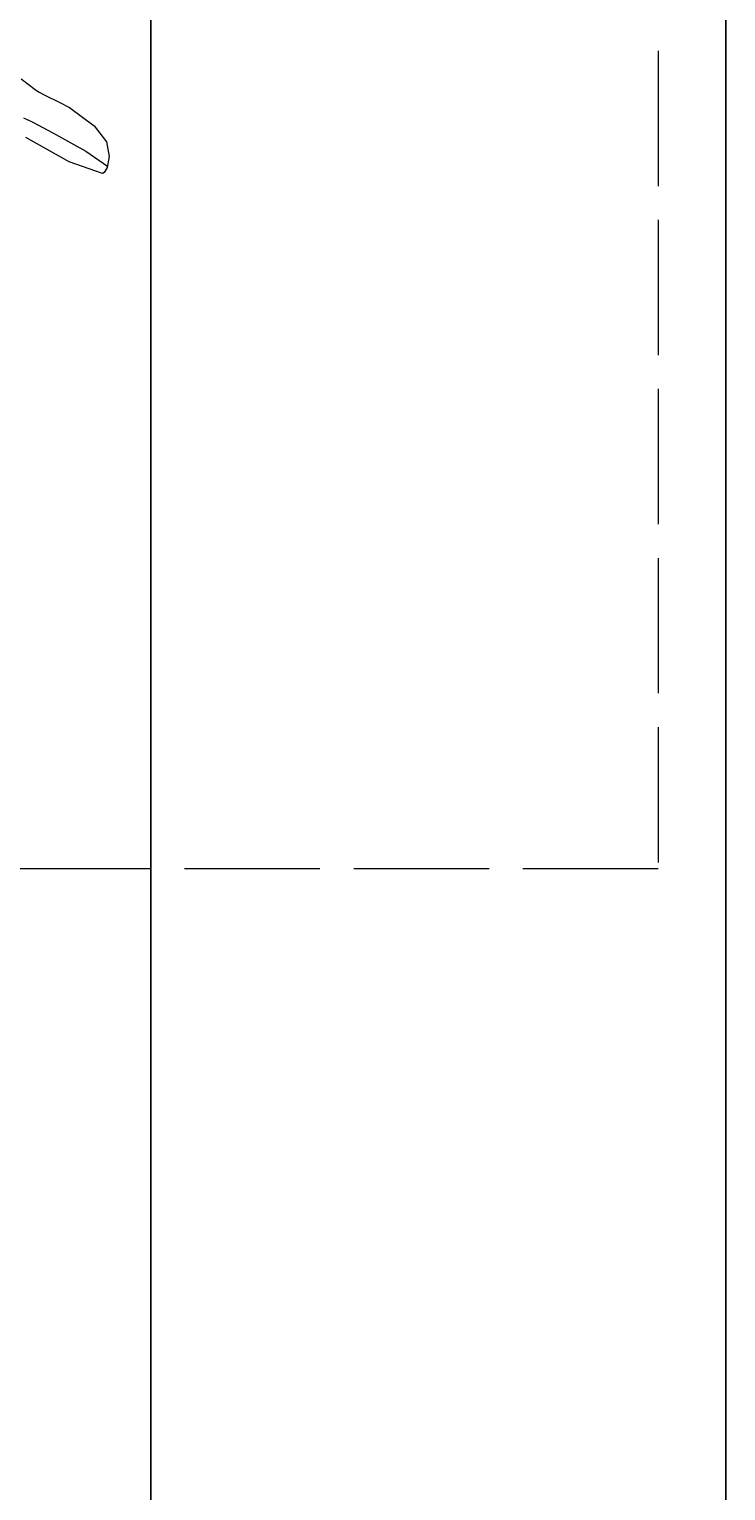
# Model space of a CAD drawing. Units: inches. Extents: x -36 to 401, y -686 to 73.
# Tile 6 of 15: x 303 to 365, y -615 to -485. Entities that reach past the tile are written whole.
import ezdxf

# ---------------------------------------------------------------- set-up
doc = ezdxf.new("R2010")
doc.units = ezdxf.units.IN
doc.header["$MEASUREMENT"] = 0
doc.linetypes.add('ACAD_ISO02W100', pattern=[15, 12, -3])
for name, color, linetype, lineweight in [('A-ANNO-DIMS', 2, 'Continuous', 18), ('A-FLOR-OVHD', 8, 'ACAD_ISO02W100', 18), ('C-PKNG-VEHI', 8, 'Continuous', 13), ('C-PROP', 7, 'Continuous', 25)]:
    doc.layers.add(name, color=color, linetype=linetype, lineweight=lineweight)
doc.styles.get("Standard").update_dxf_attribs({"font": 'arial.ttf'})
doc.dimstyles.get("Standard").update_dxf_attribs({"dimtxt": 0.18, "dimasz": 0.18, "dimexe": 0.18, "dimexo": 0.0625, "dimgap": 0.09, "dimtad": 0, "dimtih": 1, "dimtoh": 1, "dimdec": 0, "dimzin": 0, "dimdsep": 46, "dimlunit": 3, "dimtxsty": 'Standard', "dimcen": 0.09, "dimadec": 0, "dimazin": 0, "dimtfac": 1, "dimtdec": 0, "dimtofl": 0, "dimtmove": 0, "dimatfit": 3, "dimfxl": 1, "dimtolj": 1, "dimtzin": 0, "dimarcsym": 0})

# ---------------------------------------------------------------- blocks, each defined once
blk = doc.blocks.new('*D74')
at = {"layer": 'A-ANNO-DIMS', "color": 0, "lineweight": -2, "transparency": 16777216}
for p, q in [((277.69, -412.27), (277.69, -685.69)), ((313.69, -421.27), (313.69, -685.69)), ((277.87, -685.51), (295.36, -685.51)), ((313.51, -685.51), (296.02, -685.51))]:
    blk.add_line(p, q, dxfattribs=at)
at = {"layer": 'A-ANNO-DIMS', "color": 0, "transparency": 16777216}
for points in [[(277.87, -685.48), (277.87, -685.54), (277.69, -685.51)], [(313.51, -685.48), (313.51, -685.54), (313.69, -685.51)]]:
    blk.add_solid(points, dxfattribs=at)
at = {"layer": 'Defpoints', "color": 0, "transparency": 16777216}
for p in [(277.69, -412.21), (313.69, -421.21), (313.69, -685.51)]:
    blk.add_point(p, dxfattribs=at)
at = {"layer": 'A-ANNO-DIMS', "color": 0, "transparency": 16777216, "insert": (295.69, -685.51), "char_height": 0.18, "attachment_point": 5}
blk.add_mtext('\\A1;3\'-0"', dxfattribs=at)

msp = doc.modelspace()

# ---------------------------------------------------------------- linework, layer by layer
at = {"layer": 'A-FLOR-OVHD'}
for p, q in [((358.69, 7.79), (358.69, -559.77)), ((358.69, -559.77), (26.38, -559.77))]:
    msp.add_line(p, q, dxfattribs=at)
at = {"layer": 'C-PKNG-VEHI'}
for p, q in [((302.18, -489.69), (303.44, -490.64)), ((303.44, -490.64), (303.74, -490.87)), ((303.74, -490.87), (304.35, -491.17)), ((304.35, -491.17), (305.57, -491.76)), ((305.57, -491.76), (306.47, -492.24)), ((306.47, -492.24), (308.68, -493.86)), ((302.41, -493.17), (303.17, -493.53)), ((303.17, -493.53), (305, -494.48)), ((308.68, -493.86), (309.75, -495.28)), ((306.44, -497.07), (302.62, -494.92)), ((305, -494.48), (307.93, -496.12)), ((307.93, -496.12), (309.86, -497.45)), ((309.75, -495.28), (310, -496.59)), ((309.42, -498.1), (306.44, -497.07)), ((309.82, -497.56), (309.56, -498)), ((310, -496.59), (309.82, -497.56)), ((309.56, -498), (309.42, -498.1))]:
    msp.add_line(p, q, dxfattribs=at)
at = {"layer": 'C-PROP'}
msp.add_line((364.69, 31.79), (364.69, -649.21), dxfattribs=at)

# ---------------------------------------------------------------- dimensions: what is measured, and where the dimension line sits
at = {"layer": 'A-ANNO-DIMS'}
dim = msp.add_linear_dim(base=(313.69, -685.51), p1=(277.69, -412.21), p2=(313.69, -421.21), dimstyle='Standard', override={"dimdec": 1, "dimlfac": 1, "dimrnd": 0, "dimzin": 1, "dimdsep": 46, "dimlunit": 4, "dimfrac": 2}, dxfattribs=at)
dim.commit()
dim.dimension.update_dxf_attribs({"geometry": '*D74', "text_midpoint": (295.69, -685.51)})

doc.saveas('drawing.dxf')
